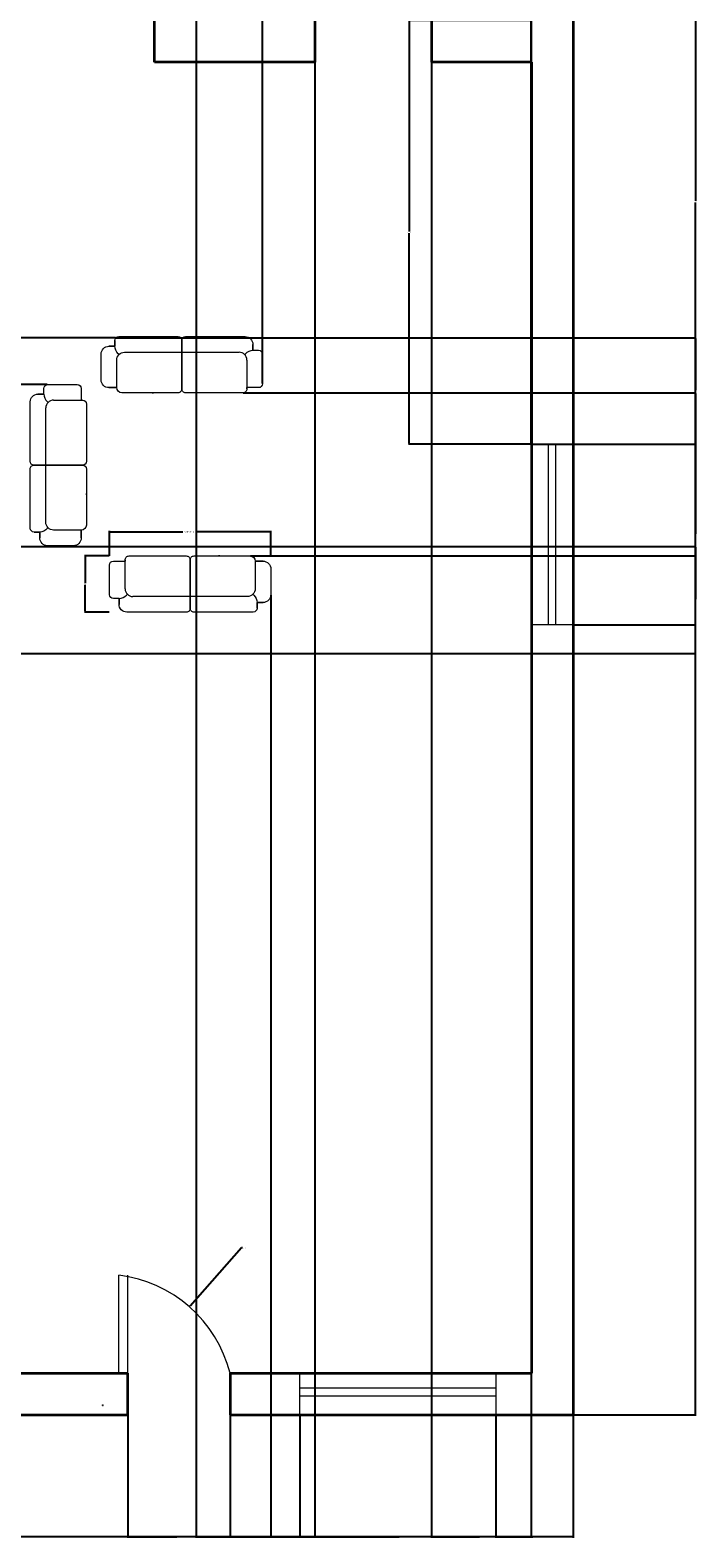
# Model space of a CAD drawing. Units: inches. Extents: x -20 to 351, y -512 to 63.
# Tile 3 of 5: x 208 to 351, y -512 to -188. Entities that reach past the tile are written whole.
import ezdxf

# ---------------------------------------------------------------- set-up
doc = ezdxf.new("R2010")
doc.units = ezdxf.units.IN
doc.header["$MEASUREMENT"] = 0
for name, color, linetype, lineweight in [('A-ANNO-DIMS', 2, 'Continuous', 18), ('A-DOOR', 3, 'Continuous', 18), ('A-FURN', 30, 'Continuous', 18), ('A-GLAZ', 4, 'Continuous', 18), ('A-WALL', 7, 'Continuous', 35)]:
    doc.layers.add(name, color=color, linetype=linetype, lineweight=lineweight)
doc.styles.get("Standard").update_dxf_attribs({"font": 'arial.ttf'})
doc.dimstyles.get("Standard").update_dxf_attribs({"dimtxt": 0.18, "dimasz": 0.18, "dimexe": 0.18, "dimexo": 0.0625, "dimgap": 0.09, "dimtad": 0, "dimtih": 1, "dimtoh": 1, "dimdec": 4, "dimzin": 0, "dimdsep": 46, "dimtxsty": 'Standard', "dimcen": 0.09, "dimadec": 0, "dimazin": 0, "dimtfac": 1, "dimtdec": 4, "dimtofl": 0, "dimtmove": 0, "dimatfit": 3, "dimfxl": 1, "dimtolj": 1, "dimtzin": 0, "dimarcsym": 0})

# ---------------------------------------------------------------- blocks, each defined once
blk = doc.blocks.new('SOFA-TWO-SEAT')
for p, q in [((2.94, 10.02), (1.68, 10.02)), ((2.94, 11.23), (2.94, 10.02)), ((17.33, 11.24), (17.33, 0.84)), ((17.33, 0.84), (17.33, 11.24)), ((32.62, 9.14), (32.62, 10.4)), ((3.35, 1.11), (3.35, 7.04)), ((3.85, 8.23), (3.67, 8.4)), ((5.03, 8.72), (17.33, 8.72)), ((17.33, 8.72), (29.64, 8.72)), ((30.82, 8.23), (30.99, 8.4)), ((31.31, 7.05), (31.31, 1.11)), ((1.68, 1.11), (3.35, 1.11)), ((10.96, 0), (11.24, 0)), ((31.31, 0.84), (31.31, 1.11))]:
    blk.add_line(p, q)
blk.add_lwpolyline([(30.47, 0), (18.17, 0, -0.414214), (17.33, 0.84, -0.414214), (16.5, 0), (11.24, 0), (11.24, 0, -0.414214), (11.24, 0), (4.45, 0, -0.404299), (3.35, 1.11), (1.68, 1.11, -0.414214), (0, 2.79), (0, 8.34, -0.414214), (1.68, 10.02), (2.94, 10.02), (2.94, 11.23, -0.409533), (3.78, 12.08), (16.5, 12.08, -0.414482), (17.33, 11.24, -0.414214), (18.17, 12.08), (30.94, 12.08, -0.414214), (32.62, 10.4), (32.62, 9.14), (33.83, 9.14, -0.394315), (34.67, 8.36), (34.67, 1.95, -0.41421), (33.83, 1.11), (31.31, 1.11), (31.31, 0.84, -0.414214), (30.47, 0, -2.414214)], format="xyb")
at = {"extrusion": (0, 0, -1)}
for centre, major_axis, start_param, end_param in [((5.45, 10.18), (-1.78, -1.78), 0, 0.723307), ((5.03, 7.04), (1.19, -1.19), 2.356194, 3.926991)]:
    blk.add_ellipse(centre, major_axis=major_axis, ratio=1, start_param=start_param, end_param=end_param, dxfattribs=at)
for centre, major_axis, start_param, end_param in [((29.64, 7.05), (1.19, -1.19), 0.785398, 2.356194), ((32.77, 6.62), (-1.78, -1.78), 3.989082, 4.712389)]:
    blk.add_ellipse(centre, major_axis=major_axis, ratio=1, start_param=start_param, end_param=end_param)
blk = doc.blocks.new('*D7')
at = {"layer": 'A-ANNO-DIMS', "color": 0, "lineweight": -2, "transparency": 16777216}
for p, q in [((224.63, -300.92), (224.63, -295.6)), ((224.81, -295.78), (240.36, -295.78)), ((259.12, -295.78), (243.57, -295.78)), ((259.3, -300.92), (259.3, -295.6))]:
    blk.add_line(p, q, dxfattribs=at)
at = {"layer": 'A-ANNO-DIMS', "color": 0, "transparency": 16777216}
for points in [[(224.81, -295.75), (224.81, -295.81), (224.63, -295.78)], [(259.12, -295.75), (259.12, -295.81), (259.3, -295.78)]]:
    blk.add_solid(points, dxfattribs=at)
at = {"layer": 'Defpoints', "color": 0, "transparency": 16777216}
for p in [(224.63, -295.78), (224.63, -300.98), (259.3, -300.98)]:
    blk.add_point(p, dxfattribs=at)
at = {"layer": 'A-ANNO-DIMS', "color": 0, "transparency": 16777216, "insert": (241.97, -295.78), "char_height": 0.18, "attachment_point": 5}
blk.add_mtext('\\A1;TWO-SEAT SOFA 35 TYP.', dxfattribs=at)
blk = doc.blocks.new('*D8')
at = {"layer": 'A-ANNO-DIMS', "color": 0, "lineweight": -2, "transparency": 16777216}
for p, q in [((224.57, -300.98), (219.25, -300.98)), ((219.43, -301.16), (219.43, -306.84)), ((219.43, -312.88), (219.43, -307.2)), ((224.57, -313.06), (219.25, -313.06))]:
    blk.add_line(p, q, dxfattribs=at)
at = {"layer": 'A-ANNO-DIMS', "color": 0, "transparency": 16777216}
for points in [[(219.4, -301.16), (219.46, -301.16), (219.43, -300.98)], [(219.4, -312.88), (219.46, -312.88), (219.43, -313.06)]]:
    blk.add_solid(points, dxfattribs=at)
at = {"layer": 'Defpoints', "color": 0, "transparency": 16777216}
for p in [(224.63, -300.98), (219.43, -313.06), (224.63, -313.06)]:
    blk.add_point(p, dxfattribs=at)
at = {"layer": 'A-ANNO-DIMS', "color": 0, "transparency": 16777216, "insert": (219.43, -307.02), "char_height": 0.18, "attachment_point": 5}
blk.add_mtext('\\A1;12 TYP.', dxfattribs=at)
blk = doc.blocks.new('*D9')
at = {"layer": 'A-ANNO-DIMS', "color": 0, "lineweight": -2, "transparency": 16777216}
for p, q in [((324.28, -315.88), (324.28, -512.19)), ((6.28, -485.83), (6.28, -512.19)), ((6.46, -512.01), (165, -512.01)), ((324.1, -512.01), (165.57, -512.01))]:
    blk.add_line(p, q, dxfattribs=at)
at = {"layer": 'A-ANNO-DIMS', "color": 0, "transparency": 16777216}
for points in [[(6.46, -511.98), (6.46, -512.04), (6.28, -512.01)], [(324.1, -511.98), (324.1, -512.04), (324.28, -512.01)]]:
    blk.add_solid(points, dxfattribs=at)
at = {"layer": 'Defpoints', "color": 0, "transparency": 16777216}
for p in [(324.28, -315.82), (6.28, -485.76), (324.28, -512.01)]:
    blk.add_point(p, dxfattribs=at)
at = {"layer": 'A-ANNO-DIMS', "color": 0, "transparency": 16777216, "insert": (165.28, -512.01), "char_height": 0.18, "attachment_point": 5}
blk.add_mtext('\\A1;318', dxfattribs=at)
blk = doc.blocks.new('*D10')
at = {"layer": 'A-ANNO-DIMS', "color": 0, "lineweight": -2, "transparency": 16777216}
for p, q in [((324.35, 36.24), (350.71, 36.24)), ((350.53, 36.06), (350.53, -224.58)), ((350.53, -485.58), (350.53, -224.95)), ((324.35, -485.76), (350.71, -485.76))]:
    blk.add_line(p, q, dxfattribs=at)
at = {"layer": 'A-ANNO-DIMS', "color": 0, "transparency": 16777216}
for points in [[(350.5, 36.06), (350.56, 36.06), (350.53, 36.24)], [(350.5, -485.58), (350.56, -485.58), (350.53, -485.76)]]:
    blk.add_solid(points, dxfattribs=at)
at = {"layer": 'Defpoints', "color": 0, "transparency": 16777216}
for p in [(324.28, 36.24), (324.28, -485.76), (350.53, -485.76)]:
    blk.add_point(p, dxfattribs=at)
at = {"layer": 'A-ANNO-DIMS', "color": 0, "transparency": 16777216, "insert": (350.53, -224.76), "char_height": 0.18, "attachment_point": 5}
blk.add_mtext('\\A1;522', dxfattribs=at)
blk = doc.blocks.new('*D25')
at = {"layer": 'A-ANNO-DIMS', "color": 0, "lineweight": -2, "transparency": 16777216}
for p, q in [((315.22, -185.76), (288.85, -185.76)), ((289.03, -185.94), (289.03, -231.17)), ((289.03, -276.76), (289.03, -231.53)), ((315.22, -276.94), (288.85, -276.94))]:
    blk.add_line(p, q, dxfattribs=at)
at = {"layer": 'A-ANNO-DIMS', "color": 0, "transparency": 16777216}
for points in [[(289, -185.94), (289.06, -185.94), (289.03, -185.76)], [(289, -276.76), (289.06, -276.76), (289.03, -276.94)]]:
    blk.add_solid(points, dxfattribs=at)
at = {"layer": 'Defpoints', "color": 0, "transparency": 16777216}
for p in [(289.03, -185.76), (315.28, -185.76), (315.28, -276.94)]:
    blk.add_point(p, dxfattribs=at)
at = {"layer": 'A-ANNO-DIMS', "color": 0, "transparency": 16777216, "insert": (289.03, -231.35), "char_height": 0.18, "attachment_point": 5}
blk.add_mtext('\\A1;91.18', dxfattribs=at)
blk = doc.blocks.new('*D26')
at = {"layer": 'A-ANNO-DIMS', "color": 0, "lineweight": -2, "transparency": 16777216}
for p, q in [((324.35, -276.94), (350.71, -276.94)), ((350.53, -277.12), (350.53, -296.2)), ((350.53, -315.64), (350.53, -296.56)), ((324.35, -315.82), (350.71, -315.82))]:
    blk.add_line(p, q, dxfattribs=at)
at = {"layer": 'A-ANNO-DIMS', "color": 0, "transparency": 16777216}
for points in [[(350.5, -277.12), (350.56, -277.12), (350.53, -276.94)], [(350.5, -315.64), (350.56, -315.64), (350.53, -315.82)]]:
    blk.add_solid(points, dxfattribs=at)
at = {"layer": 'Defpoints', "color": 0, "transparency": 16777216}
for p in [(324.28, -276.94), (324.28, -315.82), (350.53, -315.82)]:
    blk.add_point(p, dxfattribs=at)
at = {"layer": 'A-ANNO-DIMS', "color": 0, "transparency": 16777216, "insert": (350.53, -296.38), "char_height": 0.18, "attachment_point": 5}
blk.add_mtext('\\A1;38.88', dxfattribs=at)
blk = doc.blocks.new('*D27')
at = {"layer": 'A-ANNO-DIMS', "color": 0, "lineweight": -2, "transparency": 16777216}
for p, q in [((307.67, -485.83), (307.67, -512.19)), ((324.28, -485.83), (324.28, -512.19)), ((307.85, -512.01), (315.61, -512.01)), ((324.1, -512.01), (316.35, -512.01))]:
    blk.add_line(p, q, dxfattribs=at)
at = {"layer": 'A-ANNO-DIMS', "color": 0, "transparency": 16777216}
for points in [[(307.85, -511.98), (307.85, -512.04), (307.67, -512.01)], [(324.1, -511.98), (324.1, -512.04), (324.28, -512.01)]]:
    blk.add_solid(points, dxfattribs=at)
at = {"layer": 'Defpoints', "color": 0, "transparency": 16777216}
for p in [(307.67, -485.76), (324.28, -485.76), (324.28, -512.01)]:
    blk.add_point(p, dxfattribs=at)
at = {"layer": 'A-ANNO-DIMS', "color": 0, "transparency": 16777216, "insert": (315.98, -512.01), "char_height": 0.18, "attachment_point": 5}
blk.add_mtext('\\A1;16.61', dxfattribs=at)
blk = doc.blocks.new('*D28')
at = {"layer": 'A-ANNO-DIMS', "color": 0, "lineweight": -2, "transparency": 16777216}
for p, q in [((228.6, -485.83), (228.6, -512.19)), ((250.53, -485.83), (250.53, -512.19)), ((228.78, -512.01), (239.1, -512.01)), ((250.35, -512.01), (240.03, -512.01))]:
    blk.add_line(p, q, dxfattribs=at)
at = {"layer": 'A-ANNO-DIMS', "color": 0, "transparency": 16777216}
for points in [[(228.78, -511.98), (228.78, -512.04), (228.6, -512.01)], [(250.35, -511.98), (250.35, -512.04), (250.53, -512.01)]]:
    blk.add_solid(points, dxfattribs=at)
at = {"layer": 'Defpoints', "color": 0, "transparency": 16777216}
for p in [(228.6, -485.76), (250.53, -485.76), (250.53, -512.01)]:
    blk.add_point(p, dxfattribs=at)
at = {"layer": 'A-ANNO-DIMS', "color": 0, "transparency": 16777216, "insert": (239.57, -512.01), "char_height": 0.18, "attachment_point": 5}
blk.add_mtext('\\A1;21.924', dxfattribs=at)
blk = doc.blocks.new('*D29')
at = {"layer": 'A-ANNO-DIMS', "color": 0, "lineweight": -2, "transparency": 16777216}
for p, q in [((250.53, -485.83), (250.53, -512.19)), ((265.52, -485.83), (265.52, -512.19)), ((250.71, -512.01), (257.57, -512.01)), ((265.34, -512.01), (258.48, -512.01))]:
    blk.add_line(p, q, dxfattribs=at)
at = {"layer": 'A-ANNO-DIMS', "color": 0, "transparency": 16777216}
for points in [[(250.71, -511.98), (250.71, -512.04), (250.53, -512.01)], [(265.34, -511.98), (265.34, -512.04), (265.52, -512.01)]]:
    blk.add_solid(points, dxfattribs=at)
at = {"layer": 'Defpoints', "color": 0, "transparency": 16777216}
for p in [(250.53, -485.76), (265.52, -485.76), (265.52, -512.01)]:
    blk.add_point(p, dxfattribs=at)
at = {"layer": 'A-ANNO-DIMS', "color": 0, "transparency": 16777216, "insert": (258.02, -512.01), "char_height": 0.18, "attachment_point": 5}
blk.add_mtext('\\A1;14.993', dxfattribs=at)
blk = doc.blocks.new('*D30')
at = {"layer": 'A-ANNO-DIMS', "color": 0, "lineweight": -2, "transparency": 16777216}
for p, q in [((265.52, -485.83), (265.52, -512.19)), ((307.67, -485.83), (307.67, -512.19)), ((265.7, -512.01), (286.2, -512.01)), ((307.49, -512.01), (287, -512.01))]:
    blk.add_line(p, q, dxfattribs=at)
at = {"layer": 'A-ANNO-DIMS', "color": 0, "transparency": 16777216}
for points in [[(265.7, -511.98), (265.7, -512.04), (265.52, -512.01)], [(307.49, -511.98), (307.49, -512.04), (307.67, -512.01)]]:
    blk.add_solid(points, dxfattribs=at)
at = {"layer": 'Defpoints', "color": 0, "transparency": 16777216}
for p in [(265.52, -485.76), (307.67, -485.76), (307.67, -512.01)]:
    blk.add_point(p, dxfattribs=at)
at = {"layer": 'A-ANNO-DIMS', "color": 0, "transparency": 16777216, "insert": (286.6, -512.01), "char_height": 0.18, "attachment_point": 5}
blk.add_mtext('\\A1;42.15', dxfattribs=at)
blk = doc.blocks.new('*D37')
at = {"layer": 'A-ANNO-DIMS', "color": 0, "lineweight": -2, "transparency": 16777216}
for p, q in [((243.28, -125.83), (243.28, -512.19)), ((315.28, -125.83), (315.28, -512.19)), ((243.46, -512.01), (279.07, -512.01)), ((315.1, -512.01), (279.5, -512.01))]:
    blk.add_line(p, q, dxfattribs=at)
at = {"layer": 'A-ANNO-DIMS', "color": 0, "transparency": 16777216}
for points in [[(243.46, -511.98), (243.46, -512.04), (243.28, -512.01)], [(315.1, -511.98), (315.1, -512.04), (315.28, -512.01)]]:
    blk.add_solid(points, dxfattribs=at)
at = {"layer": 'Defpoints', "color": 0, "transparency": 16777216}
for p in [(243.28, -125.76), (315.28, -125.76), (315.28, -512.01)]:
    blk.add_point(p, dxfattribs=at)
at = {"layer": 'A-ANNO-DIMS', "color": 0, "transparency": 16777216, "insert": (279.28, -512.01), "char_height": 0.18, "attachment_point": 5}
blk.add_mtext('\\A1;72', dxfattribs=at)
blk = doc.blocks.new('*D45')
at = {"layer": 'A-ANNO-DIMS', "color": 0, "lineweight": -2, "transparency": 16777216}
for p, q in [((293.86, -194.83), (293.86, -512.19)), ((315.28, -194.83), (315.28, -512.19)), ((294.04, -512.01), (304.11, -512.01)), ((315.1, -512.01), (305.04, -512.01))]:
    blk.add_line(p, q, dxfattribs=at)
at = {"layer": 'A-ANNO-DIMS', "color": 0, "transparency": 16777216}
for points in [[(294.04, -511.98), (294.04, -512.04), (293.86, -512.01)], [(315.1, -511.98), (315.1, -512.04), (315.28, -512.01)]]:
    blk.add_solid(points, dxfattribs=at)
at = {"layer": 'Defpoints', "color": 0, "transparency": 16777216}
for p in [(293.86, -194.76), (315.28, -194.76), (293.86, -512.01)]:
    blk.add_point(p, dxfattribs=at)
at = {"layer": 'A-ANNO-DIMS', "color": 0, "transparency": 16777216, "insert": (304.57, -512.01), "char_height": 0.18, "attachment_point": 5}
blk.add_mtext('\\A1;21.425', dxfattribs=at)
blk = doc.blocks.new('*D46')
at = {"layer": 'A-ANNO-DIMS', "color": 0, "lineweight": -2, "transparency": 16777216}
for p, q in [((268.75, -194.83), (268.75, -512.19)), ((293.86, -194.83), (293.86, -512.19)), ((268.93, -512.01), (280.93, -512.01)), ((293.68, -512.01), (281.68, -512.01))]:
    blk.add_line(p, q, dxfattribs=at)
at = {"layer": 'A-ANNO-DIMS', "color": 0, "transparency": 16777216}
for points in [[(268.93, -511.98), (268.93, -512.04), (268.75, -512.01)], [(293.68, -511.98), (293.68, -512.04), (293.86, -512.01)]]:
    blk.add_solid(points, dxfattribs=at)
at = {"layer": 'Defpoints', "color": 0, "transparency": 16777216}
for p in [(268.75, -194.76), (293.86, -194.76), (268.75, -512.01)]:
    blk.add_point(p, dxfattribs=at)
at = {"layer": 'A-ANNO-DIMS', "color": 0, "transparency": 16777216, "insert": (281.3, -512.01), "char_height": 0.18, "attachment_point": 5}
blk.add_mtext('\\A1;25.11', dxfattribs=at)
blk = doc.blocks.new('*D48')
at = {"layer": 'A-ANNO-DIMS', "color": 0, "lineweight": -2, "transparency": 16777216}
for p, q in [((168.35, -298.93), (350.71, -298.93)), ((350.53, -299.11), (350.53, -310.27)), ((350.53, -321.78), (350.53, -310.63)), ((159.35, -321.96), (350.71, -321.96))]:
    blk.add_line(p, q, dxfattribs=at)
at = {"layer": 'A-ANNO-DIMS', "color": 0, "transparency": 16777216}
for points in [[(350.5, -299.11), (350.56, -299.11), (350.53, -298.93)], [(350.5, -321.78), (350.56, -321.78), (350.53, -321.96)]]:
    blk.add_solid(points, dxfattribs=at)
at = {"layer": 'Defpoints', "color": 0, "transparency": 16777216}
for p in [(168.28, -298.93), (159.28, -321.96), (350.53, -321.96)]:
    blk.add_point(p, dxfattribs=at)
at = {"layer": 'A-ANNO-DIMS', "color": 0, "transparency": 16777216, "insert": (350.53, -310.45), "char_height": 0.18, "attachment_point": 5}
blk.add_mtext('\\A1;23.03', dxfattribs=at)
blk = doc.blocks.new('*D62')
at = {"layer": 'A-ANNO-DIMS', "color": 0, "lineweight": -2, "transparency": 16777216}
for p, q in [((257.5, -263.86), (257.5, 62.67)), ((257.68, 62.49), (286, 62.49)), ((315.1, 62.49), (286.79, 62.49)), ((315.28, -276.88), (315.28, 62.67))]:
    blk.add_line(p, q, dxfattribs=at)
at = {"layer": 'A-ANNO-DIMS', "color": 0, "transparency": 16777216}
for points in [[(257.68, 62.52), (257.68, 62.46), (257.5, 62.49)], [(315.1, 62.52), (315.1, 62.46), (315.28, 62.49)]]:
    blk.add_solid(points, dxfattribs=at)
at = {"layer": 'Defpoints', "color": 0, "transparency": 16777216}
for p in [(315.28, 62.49), (257.5, -263.93), (315.28, -276.94)]:
    blk.add_point(p, dxfattribs=at)
at = {"layer": 'A-ANNO-DIMS', "color": 0, "transparency": 16777216, "insert": (286.39, 62.49), "char_height": 0.18, "attachment_point": 5}
blk.add_mtext('\\A1;57.78', dxfattribs=at)
blk = doc.blocks.new('*D63')
at = {"layer": 'A-ANNO-DIMS', "color": 0, "lineweight": -2, "transparency": 16777216}
for p, q in [((253.37, -265.88), (350.71, -265.88)), ((350.53, -266.06), (350.53, -283.25)), ((350.53, -300.8), (350.53, -283.61)), ((254.91, -300.98), (350.71, -300.98))]:
    blk.add_line(p, q, dxfattribs=at)
at = {"layer": 'A-ANNO-DIMS', "color": 0, "transparency": 16777216}
for points in [[(350.5, -266.06), (350.56, -266.06), (350.53, -265.88)], [(350.5, -300.8), (350.56, -300.8), (350.53, -300.98)]]:
    blk.add_solid(points, dxfattribs=at)
at = {"layer": 'Defpoints', "color": 0, "transparency": 16777216}
for p in [(253.31, -265.88), (254.85, -300.98), (350.53, -300.98)]:
    blk.add_point(p, dxfattribs=at)
at = {"layer": 'A-ANNO-DIMS', "color": 0, "transparency": 16777216, "insert": (350.53, -283.43), "char_height": 0.18, "attachment_point": 5}
blk.add_mtext('\\A1;35.1', dxfattribs=at)
blk = doc.blocks.new('*D64')
at = {"layer": 'A-ANNO-DIMS', "color": 0, "lineweight": -2, "transparency": 16777216}
for p, q in [((259.3, -309.39), (259.3, -512.19)), ((315.28, -315.88), (315.28, -512.19)), ((259.48, -512.01), (286.9, -512.01)), ((315.1, -512.01), (287.69, -512.01))]:
    blk.add_line(p, q, dxfattribs=at)
at = {"layer": 'A-ANNO-DIMS', "color": 0, "transparency": 16777216}
for points in [[(259.48, -511.98), (259.48, -512.04), (259.3, -512.01)], [(315.1, -511.98), (315.1, -512.04), (315.28, -512.01)]]:
    blk.add_solid(points, dxfattribs=at)
at = {"layer": 'Defpoints', "color": 0, "transparency": 16777216}
for p in [(259.3, -309.32), (315.28, -315.82), (315.28, -512.01)]:
    blk.add_point(p, dxfattribs=at)
at = {"layer": 'A-ANNO-DIMS', "color": 0, "transparency": 16777216, "insert": (287.29, -512.01), "char_height": 0.18, "attachment_point": 5}
blk.add_mtext('\\A1;55.98', dxfattribs=at)
blk = doc.blocks.new('*D65')
at = {"layer": 'A-ANNO-DIMS', "color": 0, "lineweight": -2, "transparency": 16777216}
for p, q in [((225.95, -254.05), (-20.15, -254.05)), ((-19.97, -254.23), (-19.97, -258.9)), ((-19.97, -263.93), (-19.97, -259.26)), ((211.25, -264.11), (-20.15, -264.11))]:
    blk.add_line(p, q, dxfattribs=at)
at = {"layer": 'A-ANNO-DIMS', "color": 0, "transparency": 16777216}
for points in [[(-20, -254.23), (-19.94, -254.23), (-19.97, -254.05)], [(-20, -263.93), (-19.94, -263.93), (-19.97, -264.11)]]:
    blk.add_solid(points, dxfattribs=at)
at = {"layer": 'Defpoints', "color": 0, "transparency": 16777216}
for p in [(-19.97, -254.05), (226.02, -254.05), (211.31, -264.11)]:
    blk.add_point(p, dxfattribs=at)
at = {"layer": 'A-ANNO-DIMS', "color": 0, "transparency": 16777216, "insert": (-19.97, -259.08), "char_height": 0.18, "attachment_point": 5}
blk.add_mtext('\\A1;10.056', dxfattribs=at)
blk = doc.blocks.new('*D66')
at = {"layer": 'A-ANNO-DIMS', "color": 0, "lineweight": -2, "transparency": 16777216}
for p, q in [((226.08, -254.05), (350.71, -254.05)), ((350.53, -254.23), (350.53, -265.31)), ((350.53, -276.76), (350.53, -265.68)), ((315.35, -276.94), (350.71, -276.94))]:
    blk.add_line(p, q, dxfattribs=at)
at = {"layer": 'A-ANNO-DIMS', "color": 0, "transparency": 16777216}
for points in [[(350.5, -254.23), (350.56, -254.23), (350.53, -254.05)], [(350.5, -276.76), (350.56, -276.76), (350.53, -276.94)]]:
    blk.add_solid(points, dxfattribs=at)
at = {"layer": 'Defpoints', "color": 0, "transparency": 16777216}
for p in [(226.02, -254.05), (350.53, -254.05), (315.28, -276.94)]:
    blk.add_point(p, dxfattribs=at)
at = {"layer": 'A-ANNO-DIMS', "color": 0, "transparency": 16777216, "insert": (350.53, -265.5), "char_height": 0.18, "attachment_point": 5}
blk.add_mtext('\\A1;22.89', dxfattribs=at)
blk = doc.blocks.new('*D81')
at = {"layer": 'A-ANNO-DIMS', "color": 0, "lineweight": -2, "transparency": 16777216}
for p, q in [((253.01, -449.83), (241.95, -462.39)), ((253.19, -449.83), (253.01, -449.83)), ((223.11, -483.67), (223.29, -483.67)), ((223.2, -483.76), (223.2, -483.58))]:
    blk.add_line(p, q, dxfattribs=at)
at = {"layer": 'A-ANNO-DIMS', "color": 0, "transparency": 16777216}
blk.add_solid([(241.93, -462.37), (241.97, -462.41), (241.83, -462.52)], dxfattribs=at)
at = {"layer": 'Defpoints', "color": 0, "transparency": 16777216}
for p in [(241.83, -462.52), (223.2, -483.67)]:
    blk.add_point(p, dxfattribs=at)
at = {"layer": 'A-ANNO-DIMS', "color": 0, "transparency": 16777216, "insert": (253.74, -449.83), "char_height": 0.18, "attachment_point": 5}
blk.add_mtext('\\A1;R28.186', dxfattribs=at)

msp = doc.modelspace()

# ---------------------------------------------------------------- linework, layer by layer
at = {"layer": 'A-DOOR'}
for p, q in [((226.604, -476.7646), (226.604, -455.694)), ((228.604, -476.7646), (228.604, -455.694))]:
    msp.add_line(p, q, dxfattribs=at)
msp.add_arc((223.2022, -483.6738), 28.1858, 14.18946, 83.067952, dxfattribs=at)
at = {"layer": 'A-FURN'}
for p, q in [((210.5323, -266.1561), (209.2669, -266.1561)), ((210.9444, -281.4383), (210.9444, -269.1367)), ((211.4357, -267.9505), (211.2644, -267.7792)), ((212.6219, -267.4592), (218.5538, -267.4592)), ((218.8286, -267.4592), (218.5538, -267.4592)), ((208.4282, -281.4383), (218.8286, -281.4383)), ((218.8286, -281.4383), (208.4282, -281.4383)), ((210.95, -293.74), (210.9444, -281.4383)), ((219.6674, -287.8081), (219.6674, -287.5333)), ((211.4413, -294.9262), (211.27, -295.0975)), ((208.4337, -295.8345), (209.6469, -295.8345)), ((209.6469, -295.8296), (209.6469, -297.095)), ((218.5538, -295.4175), (212.6275, -295.4175)), ((218.5538, -297.095), (218.5538, -295.4175))]:
    msp.add_line(p, q, dxfattribs=at)
msp.add_lwpolyline([(219.6674, -268.2979), (219.6674, -280.5996, -0.41421356), (218.8286, -281.4383, -0.41421356), (219.6674, -282.2771), (219.6674, -287.5333), (219.6674, -287.5333, -0.41421356), (219.6674, -287.5333), (219.6674, -294.3211, -0.40429871), (218.5538, -295.4175), (218.5538, -297.095, -0.41421356), (216.8763, -298.7725), (211.3244, -298.7725, -0.41421356), (209.6469, -297.095), (209.6469, -295.8345), (208.4337, -295.8345, -0.40953287), (207.5894, -294.9957), (207.5894, -282.2771, -0.4144824), (208.4282, -281.4383, -0.41421356), (207.5894, -280.5996), (207.5894, -267.8336, -0.41421356), (209.2669, -266.1561), (210.5274, -266.1561), (210.5274, -264.9429, -0.39431507), (211.3088, -264.1062), (217.715, -264.1042, -0.41421005), (218.5538, -264.9429), (218.5538, -267.4592), (218.8286, -267.4592, -0.41421356), (219.6674, -268.2979, -2.41421356)], format="xyb", dxfattribs=at)
for centre, major_axis, start_param, end_param in [((213.0437, -266), (1.7793, -1.7793), 3.98908175, 4.71238898), ((212.6219, -269.1367), (1.1862, 1.1862), 0.78539816, 2.35619449)]:
    msp.add_ellipse(centre, major_axis=major_axis, ratio=1, start_param=start_param, end_param=end_param, dxfattribs=at)
at = {"layer": 'A-FURN', "extrusion": (0, 0, -1)}
for centre, major_axis, start_param, end_param in [((209.4907, -293.3182), (1.7793, -1.7793), 0, 0.72330723), ((212.6275, -293.74), (1.1862, 1.1862), 2.35619449, 3.92699082)]:
    msp.add_ellipse(centre, major_axis=major_axis, ratio=1, start_param=start_param, end_param=end_param, dxfattribs=at)
at = {"layer": 'A-GLAZ'}
for p, q in [((318.8925, -276.9398), (318.8925, -315.8223)), ((320.4509, -276.9398), (320.4509, -315.8223)), ((307.6737, -480.0314), (265.5208, -480.0314)), ((307.6737, -481.6952), (265.5208, -481.6952))]:
    msp.add_line(p, q, dxfattribs=at)
for points in [[(315.2844, -276.9398), (324.2844, -276.9398), (324.2844, -315.8223), (315.2844, -315.8223)], [(307.6737, -476.7646), (307.6737, -485.7646), (265.5208, -485.7646), (265.5208, -476.7646)]]:
    msp.add_lwpolyline(points, close=True, dxfattribs=at)
at = {"layer": 'A-WALL'}
for p, q in [((324.2844, 36.2354), (324.2844, -485.7646)), ((234.2844, -194.7646), (234.2844, -125.7646)), ((268.7509, -185.7646), (268.7509, -194.7646)), ((293.8591, -185.7646), (293.8591, -194.7646)), ((268.7509, -194.7646), (234.2844, -194.7646)), ((315.2844, -194.7646), (293.8591, -194.7646)), ((315.2844, -194.7646), (315.2844, -476.7646)), ((15.2844, -476.7646), (228.604, -476.7646)), ((228.604, -485.7646), (228.604, -476.7646)), ((250.5281, -476.7646), (250.5281, -485.7646)), ((250.5281, -476.7646), (315.2844, -476.7646)), ((6.2844, -485.7646), (228.604, -485.7646)), ((250.5281, -485.7646), (324.2844, -485.7646))]:
    msp.add_line(p, q, dxfattribs=at)

# ---------------------------------------------------------------- block references
at = {"layer": 'A-FURN'}
msp.add_blockref('SOFA-TWO-SEAT', (222.833, -265.878), dxfattribs=at)
at = {"layer": 'A-FURN', "rotation": 180}
msp.add_blockref('SOFA-TWO-SEAT', (259.2993, -300.9812), dxfattribs=at)

# ---------------------------------------------------------------- dimensions: what is measured, and where the dimension line sits
at = {"layer": 'A-ANNO-DIMS'}
for base, p1, p2, override, picture, middle in [((315.2844, 62.4854), (257.501, -263.9256), (315.2844, -276.9398), {"dimdec": 2, "dimlfac": 1, "dimrnd": 0, "dimzin": 0, "dimdsep": 46, "dimlunit": 2}, '*D62', (286.3927, 62.4854)), ((315.2844, -512.0146), (243.2844, -125.7646), (315.2844, -125.7646), {"dimdec": 0, "dimlfac": 1, "dimrnd": 0, "dimzin": 0, "dimdsep": 46, "dimlunit": 2}, '*D37', (279.2844, -512.0146)), ((268.7509, -512.0146), (293.8591, -194.7646), (268.7509, -194.7646), {"dimdec": 2, "dimlfac": 1, "dimrnd": 0, "dimzin": 0, "dimdsep": 46, "dimlunit": 2}, '*D46', (281.305, -512.0146)), ((293.8591, -512.0146), (315.2844, -194.7646), (293.8591, -194.7646), {"dimdec": 3, "dimlfac": 1, "dimrnd": 0, "dimzin": 0, "dimdsep": 46, "dimlunit": 2}, '*D45', (304.5718, -512.0146)), ((315.2844, -512.0146), (259.2995, -309.3243), (315.2844, -315.8223), {"dimdec": 2, "dimlfac": 1, "dimrnd": 0, "dimzin": 0, "dimdsep": 46, "dimlunit": 2}, '*D64', (287.292, -512.0146)), ((324.2844, -512.0146), (6.2844, -485.7646), (324.2844, -315.8223), {"dimdec": 0, "dimlfac": 1, "dimrnd": 0, "dimzin": 0, "dimdsep": 46, "dimlunit": 2}, '*D9', (165.2844, -512.0146)), ((250.5281, -512.0146), (228.604, -485.7646), (250.5281, -485.7646), {"dimdec": 3, "dimlfac": 1, "dimrnd": 0, "dimzin": 0, "dimdsep": 46, "dimlunit": 2}, '*D28', (239.566, -512.0146)), ((265.5208, -512.0146), (250.5281, -485.7646), (265.5208, -485.7646), {"dimdec": 3, "dimlfac": 1, "dimrnd": 0, "dimzin": 0, "dimdsep": 46, "dimlunit": 2}, '*D29', (258.0245, -512.0146)), ((307.6737, -512.0146), (265.5208, -485.7646), (307.6737, -485.7646), {"dimdec": 2, "dimlfac": 1, "dimrnd": 0, "dimzin": 0, "dimdsep": 46, "dimlunit": 2}, '*D30', (286.5973, -512.0146)), ((324.2844, -512.0146), (307.6737, -485.7646), (324.2844, -485.7646), {"dimdec": 2, "dimlfac": 1, "dimrnd": 0, "dimzin": 0, "dimdsep": 46, "dimlunit": 2}, '*D27', (315.9791, -512.0146))]:
    dim = msp.add_linear_dim(base=base, p1=p1, p2=p2, dimstyle='Standard', override=override, dxfattribs=at)
    dim.commit()
    dim.dimension.update_dxf_attribs({"geometry": picture, "text_midpoint": middle})
for base, p1, p2, override, picture, middle in [((350.5345, -485.7646), (324.2844, 36.2354), (324.2844, -485.7646), {"dimdec": 0, "dimlfac": 1, "dimrnd": 0, "dimzin": 0, "dimdsep": 46, "dimlunit": 2}, '*D10', (350.5345, -224.7646)), ((289.0345, -185.7646), (315.2844, -276.9398), (315.2844, -185.7646), {"dimdec": 2, "dimlfac": 1, "dimrnd": 0, "dimzin": 0, "dimdsep": 46, "dimlunit": 2}, '*D25', (289.0345, -231.3522)), ((-19.9656, -254.0504), (211.3088, -264.1062), (226.0172, -254.0504), {"dimdec": 3, "dimlfac": 1, "dimrnd": 0, "dimzin": 0, "dimdsep": 46, "dimlunit": 2}, '*D65', (-19.9656, -259.0783)), ((350.5345, -254.0504), (315.2844, -276.9398), (226.0172, -254.0504), {"dimdec": 2, "dimlfac": 1, "dimrnd": 0, "dimzin": 0, "dimdsep": 46, "dimlunit": 2}, '*D66', (350.5345, -265.4951)), ((350.5345, -300.9813), (253.3073, -265.8779), (254.8482, -300.9813), {"dimdec": 1, "dimlfac": 1, "dimrnd": 0, "dimzin": 0, "dimdsep": 46, "dimlunit": 2}, '*D63', (350.5345, -283.4296)), ((350.5345, -315.8223), (324.2844, -276.9398), (324.2844, -315.8223), {"dimdec": 2, "dimlfac": 1, "dimrnd": 0, "dimzin": 0, "dimdsep": 46, "dimlunit": 2}, '*D26', (350.5345, -296.3811)), ((350.5345, -321.9646), (168.2844, -298.9325), (159.2844, -321.9646), {"dimdec": 2, "dimlfac": 1, "dimrnd": 0, "dimzin": 0, "dimdsep": 46, "dimlunit": 2}, '*D48', (350.5345, -310.4485))]:
    dim = msp.add_linear_dim(base=base, p1=p1, p2=p2, angle=90, dimstyle='Standard', override=override, dxfattribs=at)
    dim.commit()
    dim.dimension.update_dxf_attribs({"geometry": picture, "text_midpoint": middle})
for base, p1, p2, angle, text, picture, middle in [((224.6312, -295.781), (259.2995, -300.9813), (224.6312, -300.9813), 180, 'TWO-SEAT SOFA <> TYP.', '*D7', (241.9654, -295.781)), ((219.431, -313.0593), (224.6312, -300.9813), (224.6312, -313.0593), 270, '<> TYP.', '*D8', (219.431, -307.0203))]:
    dim = msp.add_linear_dim(base=base, p1=p1, p2=p2, angle=angle, text=text, dimstyle='Standard', override={"dimdec": 0, "dimlfac": 1, "dimrnd": 0, "dimzin": 0, "dimdsep": 46, "dimlunit": 2}, dxfattribs=at)
    dim.commit()
    dim.dimension.update_dxf_attribs({"geometry": picture, "text_midpoint": middle})
dim = msp.add_radius_dim(center=(223.2022, -483.6738), mpoint=(241.8311, -462.5219), dimstyle='Standard', override={"dimdec": 3, "dimlfac": 1, "dimrnd": 0, "dimzin": 0, "dimdsep": 46, "dimlunit": 2}, dxfattribs=at)
dim.commit()
dim.dimension.update_dxf_attribs({"geometry": '*D81', "text_midpoint": (253.7382, -449.8307), "dimtype": 164})

doc.saveas('drawing.dxf')
